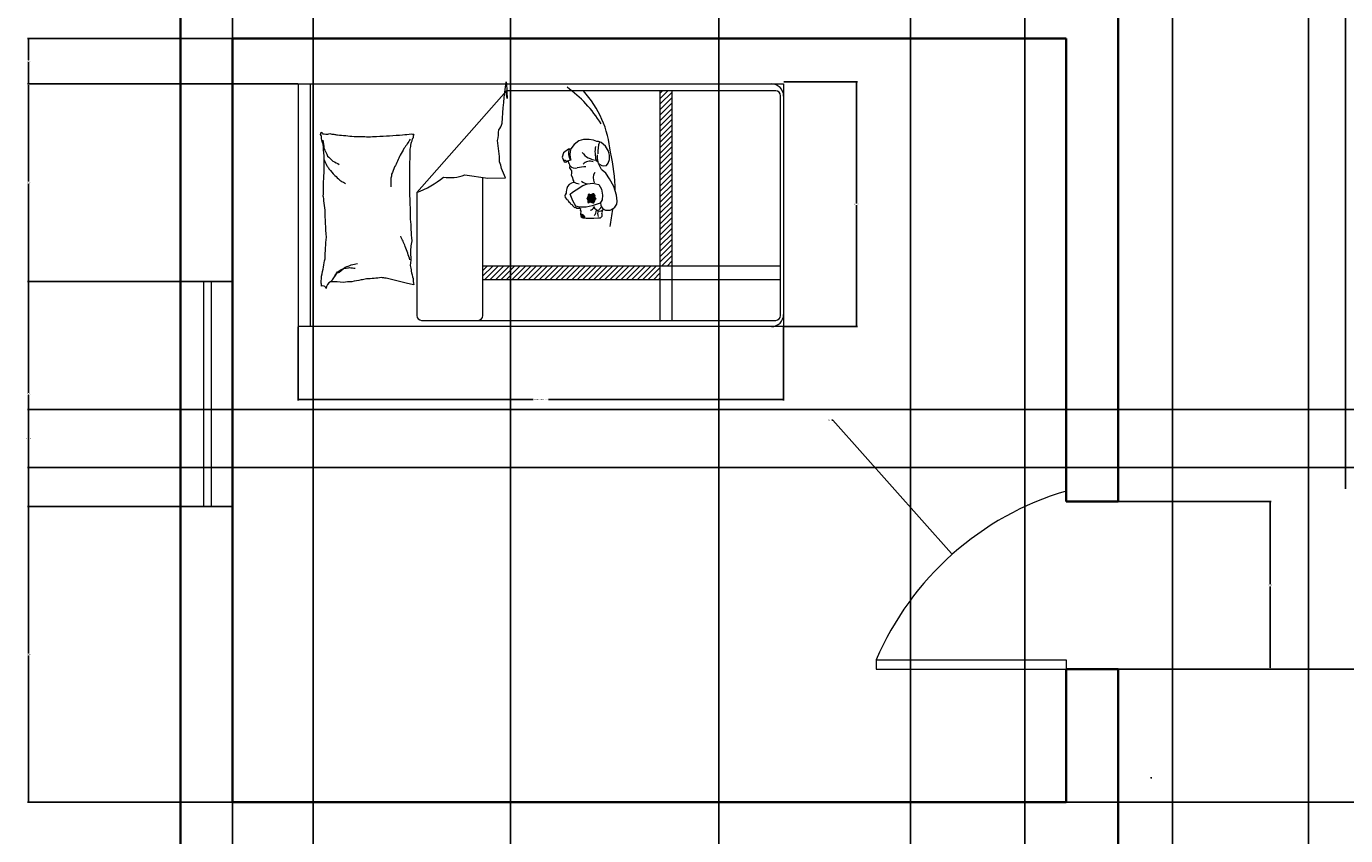
# Model space of a CAD drawing. Units: inches. Extents: x -20 to 351, y -512 to 63.
# Tile 2 of 5: x -20 to 208, y -328 to -188. Entities that reach past the tile are written whole.
import ezdxf

# ---------------------------------------------------------------- set-up
doc = ezdxf.new("R2010")
doc.units = ezdxf.units.IN
doc.header["$MEASUREMENT"] = 0
for name, color, linetype, lineweight in [('A-ANNO-DIMS', 2, 'Continuous', 18), ('A-DOOR', 3, 'Continuous', 18), ('A-FURN', 30, 'Continuous', 18), ('A-GLAZ', 4, 'Continuous', 18), ('A-WALL', 7, 'Continuous', 35)]:
    doc.layers.add(name, color=color, linetype=linetype, lineweight=lineweight)
doc.styles.get("Standard").update_dxf_attribs({"font": 'arial.ttf'})
doc.dimstyles.get("Standard").update_dxf_attribs({"dimtxt": 0.18, "dimasz": 0.18, "dimexe": 0.18, "dimexo": 0.0625, "dimgap": 0.09, "dimtad": 0, "dimtih": 1, "dimtoh": 1, "dimdec": 4, "dimzin": 0, "dimdsep": 46, "dimtxsty": 'Standard', "dimcen": 0.09, "dimadec": 0, "dimazin": 0, "dimtfac": 1, "dimtdec": 4, "dimtofl": 0, "dimtmove": 0, "dimatfit": 3, "dimfxl": 1, "dimtolj": 1, "dimtzin": 0, "dimarcsym": 0})
pattern_1 = [(135, (-420.77409, 493.76136), (-0.08072188, -0.08072188), [])]

# ---------------------------------------------------------------- blocks, each defined once
blk = doc.blocks.new('BED-SINGLE')
h = blk.add_hatch()
h.set_pattern_fill('ANSI31', color=256, scale=0.209657, angle=90, style=0)
h.set_pattern_definition([(225, (-28.8794, 49.6857), (-0.4706923, 0.4706923), [])])
h.paths.add_polyline_path([(62.56, 8.11), (62.56, 10.46), (31.92, 10.46), (31.92, 8.11)])
h.paths.add_polyline_path([(64.62, 10.46), (64.62, 40.74), (62.56, 40.74), (62.56, 10.46)])
h = blk.add_hatch()
h.set_pattern_fill('ANSI31', color=256, scale=0.913264, angle=90, style=0)
h.set_pattern_definition(pattern_1)
h.paths.add_polyline_path([(51.28, 22.35), (51.3, 22.58), (51.22, 22.8), (51.07, 22.92), (50.9, 22.92), (50.65, 22.81), (50.46, 22.77), (50.38, 22.84), (50.26, 22.89), (50.12, 22.84), (50.1, 22.73), (50.1, 22.6), (50.04, 22.43), (49.91, 22.22), (49.88, 22.16), (50.03, 21.91), (50.07, 21.8), (50.04, 21.63), (50.02, 21.51), (50.13, 21.39), (50.25, 21.43), (50.34, 21.55), (50.56, 21.53), (50.93, 21.38), (51.11, 21.41), (51.13, 21.53), (51.16, 21.62), (51.25, 21.7), (51.25, 21.79), (51.3, 21.95), (51.4, 22.06), (51.46, 22.11), (51.37, 22.18)])
h = blk.add_hatch()
h.set_pattern_fill('ANSI31', color=256, scale=0.913264, angle=90, style=0)
h.set_pattern_definition(pattern_1)
h.paths.add_polyline_path([(48.8, 19.38), (48.81, 19.17), (48.88, 18.99), (49.05, 18.85), (49.19, 18.79), (49.55, 18.75, 0.479357)])
for p, q in [((0, 41.93), (83.86, 41.93)), ((83.86, 41.93), (83.86, 0)), ((20.48, 23.17), (35.99, 40.74)), ((82.51, 40.74), (35.99, 40.74)), ((62.56, 1.08), (62.56, 40.74)), ((64.62, 1.08), (64.62, 40.74)), ((83.35, 1.92), (83.35, 39.9)), ((31.92, 1.92), (31.92, 25.76)), ((20.48, 23.17), (20.48, 1.92)), ((83.86, 0), (0, 0)), ((21.32, 1.08), (82.51, 1.08))]:
    blk.add_line(p, q)
for points in [[(0, 41.93), (0, 0)], [(2.1, 0), (2.1, 41.93)], [(49.88, 18.74), (50.44, 18.72), (51.09, 18.75), (51.78, 18.78), (51.99, 18.81), (52.24, 18.82), (52.5, 19.09), (52.51, 19.35), (52.46, 19.55), (52.59, 19.75), (52.54, 19.93), (52.68, 20.27), (52.85, 20.24), (53.09, 20.11), (53.92, 20.14), (54.4, 20.39), (54.7, 20.65), (55.03, 21.16), (55.11, 21.69), (54.99, 22.73), (54.51, 24.21), (53.78, 25.53), (53.17, 26.52), (52.53, 27.05), (52.38, 27.16), (51.98, 27.94), (51.97, 28.02), (52.04, 28.1), (52.44, 27.84), (52.72, 27.76), (53.28, 27.82), (53.58, 28.27), (53.78, 28.87), (53.81, 29.61), (53.61, 30.34), (53.08, 31.16), (52.32, 31.81), (51.86, 31.98), (51.61, 32), (51.05, 32.23), (50.29, 32.34), (49.27, 32.34), (48.48, 32.12), (47.69, 31.5), (47.1, 30.74), (46.7, 30.65), (45.83, 30.03), (45.63, 29.27), (45.94, 28.45), (46.23, 28.39), (46.51, 28.63), (46.59, 28.65), (46.7, 28.38), (46.79, 28.19), (46.84, 28.15), (46.88, 27.91), (46.94, 27.83), (46.9, 27.43), (47.08, 27.07), (47.21, 26.95), (47.22, 26.46), (47.16, 26.24), (47.34, 25.81), (47.42, 25.77), (47.46, 25.38), (47.62, 25.1), (47.53, 24.92), (47.25, 24.78), (46.82, 24.56), (46.52, 24.21), (46.42, 23.85), (46.36, 23.64), (46.33, 23.32), (46.29, 23.08), (46.15, 22.79), (46.09, 22.63), (46.1, 22.34), (46.39, 21.98), (46.55, 21.94), (46.69, 21.61), (46.82, 21.43), (46.98, 21.37), (47.06, 21.28), (47.13, 21.18), (47.37, 21.06), (47.42, 21.02), (47.42, 20.94), (47.65, 20.72), (47.76, 20.61), (47.94, 20.63), (48.13, 20.48), (48.29, 20.49), (48.59, 20.46), (48.72, 20.43), (48.78, 20.4), (48.76, 20.33), (48.74, 20.13), (48.82, 19.97), (48.83, 19.89), (48.79, 19.52), (48.81, 19.17), (48.88, 18.99), (49.05, 18.85), (49.19, 18.79), (49.73, 18.74), (49.88, 18.74)], [(47.98, 20.81), (47.46, 21.73), (46.99, 22.87), (47.37, 23.23), (48.03, 23.64), (49.19, 24.37), (50.01, 24.7), (50.89, 24.79), (51.92, 24.54), (52.4, 23.78), (52.6, 22.7), (52.51, 21.89), (52.18, 21.31), (50.82, 20.9), (49.74, 20.66), (48.6, 20.63), (47.98, 20.81)], [(49.88, 22.16), (50.03, 21.91), (50.07, 21.8), (50.04, 21.63), (50.02, 21.51), (50.13, 21.39), (50.25, 21.43), (50.34, 21.55), (50.56, 21.53), (50.93, 21.38), (51.11, 21.41), (51.13, 21.53), (51.16, 21.62), (51.25, 21.7), (51.25, 21.79), (51.3, 21.95), (51.4, 22.06), (51.46, 22.11), (51.37, 22.18), (51.28, 22.35), (51.3, 22.58), (51.22, 22.8), (51.07, 22.92), (50.9, 22.92), (50.65, 22.81), (50.46, 22.77), (50.38, 22.84), (50.26, 22.89), (50.12, 22.84), (50.1, 22.73), (50.1, 22.6), (50.04, 22.43), (49.91, 22.22), (49.88, 22.16)], [(83.35, 10.46), (31.92, 10.46)], [(83.35, 8.11), (31.92, 8.11)]]:
    blk.add_lwpolyline(points)
for points in [[(35.81, 25.72, 0.027362), (35.12, 27.33, 0.040834), (34.81, 28.47, 0.038441), (34.42, 32.14, 0.076528), (34.64, 34, 0.103649), (35.24, 35.15, -0.018778), (35.94, 42.28, -0.024037), (36.09, 39.44, -0.052315), (35.99, 40.74)], [(5.6, 7.76, 0.263368), (4.81, 6.59, 0.494818), (4.03, 6.97, 0.049225), (3.96, 7.71, 0.036831), (4.03, 8.71, 0.031893), (4.37, 10.3, -0.035782), (4.66, 11.72, -0.032941), (4.91, 15.48, -0.026564), (4.66, 20.14, -0.017905), (4.44, 21.72, 0.033397), (4.34, 22.56, 0.03204), (4.37, 24.12, -0.018442), (4.5, 26.82, -0.010837), (4.47, 29.53, -0.014624), (4.34, 31.54, -0.111249), (4.04, 32.49, 0.153708), (3.87, 33.19, 0.076444), (3.94, 33.51, 0.215512), (4.03, 33.59, 0.585858), (4.16, 33.48, -0.363489), (4.26, 33.27, -0.191716), (4.75, 33.27, 0.129675), (5.45, 33.35, 0.01735), (6.15, 33.23, -0.019326), (6.78, 33.12, -0.018818), (9.65, 32.84, -0.021828), (12.13, 32.8, -0.006204), (13.55, 32.86, -0.001963), (18.04, 33.12, -0.028341), (19.55, 33.29, 0.117014), (19.92, 33.27, 0.36606), (19.96, 33.21, 0.03973), (19.84, 32.64, 0.048309), (19.62, 32.07, -0.062981), (19.45, 31.62, -0.04058), (19.31, 30.64, -0.014345), (19.22, 27.84, -0.005484), (19.25, 22.58, -0.007153), (19.37, 18.55, -0.008762), (19.49, 16.76, 0.008153), (19.61, 14.85, 0.06251), (19.42, 12.45, -0.078669), (19.34, 10.54, -0.047825), (19.54, 9.6, 0.034494), (19.84, 8.31, 0.023571), (19.97, 7.25, 0.510228), (19.92, 7.21), (18.66, 7.52), (15.2, 8.39, -0.073041), (14.38, 8.47, -0.023305), (11.82, 8.23, -0.018299), (10.86, 8.06, 0.01097), (9.27, 7.75, 0.042281), (7.83, 7.63, 0.027201), (5.59, 7.75)], [(4.26, 32.24, -0.088153), (4.41, 30.79, -0.088153), (5.05, 29.48, -0.077547), (5.96, 28.58, -0.077547), (7.1, 27.99)], [(19.37, 32.4, -0.016108), (18.27, 30.77, -0.024599), (17.64, 29.64, -0.009477), (16.66, 27.59, -0.015937), (16.15, 26.34, -0.072521), (16, 25.65, -0.033339), (15.99, 24.13)], [(4.5, 28.8, -0.027842), (4.95, 27.81, -0.048685), (5.29, 27.28, -0.023666), (6.31, 26.11, -0.031223), (7.18, 25.31, -0.046801), (7.5, 25.1, -0.023191), (8.2, 24.76)], [(20.48, 23.17, 0.085272), (25.1, 25.83, 0.124044), (28.77, 26.21), (32.77, 25.64), (35.81, 25.72)], [(19.31, 11.55, -0.009729), (18.93, 12.7, -0.009729), (18.51, 13.82, -0.007971), (18.13, 14.74, -0.007971), (17.72, 15.64)], [(5.6, 7.75, 0.077379), (6.66, 9.21, 0.077379), (8.12, 10.28, 0.047525), (9.15, 10.7, 0.047525), (10.25, 10.91)], [(6.27, 8.86, 0.05369), (6.82, 9.46, 0.070312), (7.33, 9.8, 0.015448), (7.69, 9.96, 0.013244), (8.12, 10.11, 0.082127), (8.88, 10.24, 0.064164), (9.85, 10.11)]]:
    blk.add_lwpolyline(points, format="xyb")
for centre, radius, start, end in [((33.6, 23.46), 22.04, 31.7708, 54.3375), ((81.77, 39.84), 2.1, 0, 90), ((35.62, 28.39), 18.42, 5.4641, 42.1092), ((82.51, 39.9), 0.839, 0, 90), ((48.38, 29.88), 1.69, 151.149, 221.3836), ((49.8, 29.77), 2.87, 160.3319, 200.5181), ((51.72, 32.02), 3.26, 215.9219, 265.4055), ((57.03, 30.22), 5.75, 171.0084, 194.554), ((54.62, 29.31), 2.97, 172.9692, 196.7988), ((56.22, 30.19), 4.47, 157.6837, 184.5902), ((27.13, 23.57), 27.62, 359.7962, 13.7616), ((46.52, 29.27), 0.673, 218.3031, 258.9374), ((47.06, 28.21), 0.555, 83.9542, 141.018), ((47.86, 28.52), 1.15, 217.108, 288.2435), ((49.63, 21.97), 5.63, 89.2848, 104.5089), ((50.34, 27.01), 1.56, 67.4286, 136.0363), ((50.26, 27.3), 1.9, 23.4063, 50.8909), ((50.11, 26.41), 1.71, 226.7949, 266.7156), ((52.75, 25.69), 1.78, 147.515, 207.2356), ((50.24, 30.81), 6.38, 245.3415, 254.4913), ((50.34, 21.04), 0.905, 279.9605, 331.843), ((52.62, 21.72), 1.86, 210.5886, 253.4912), ((51.62, 20.94), 0.779, 295.2148, 339.8011), ((53.63, 21.39), 1.39, 182.1498, 236.1783), ((48.92, 18.76), 0.631, 359.0987, 101.5429), ((50.37, 20.09), 1.16, 309.7451, 1.7337), ((53.53, 19.57), 1.79, 164.8422, 197.2397), ((52.13, 20.47), 0.53, 266.1994, 319.0666), ((12.56, 24.85), 42.04, 349.6217, 353.7472), ((21.32, 1.92), 0.839, 180, 270), ((31.08, 1.92), 0.839, 270, 0), ((81.77, 2.1), 2.1, 270, 0), ((82.51, 1.92), 0.839, 270, 0)]:
    blk.add_arc(centre, radius, start, end)
blk = doc.blocks.new('*D5')
at = {"layer": 'A-ANNO-DIMS', "color": 0, "lineweight": -2, "transparency": 16777216}
for p, q in [((26.62, -239.81), (26.62, -252.51)), ((110.48, -239.81), (110.48, -252.51)), ((26.8, -252.33), (67.23, -252.33)), ((110.3, -252.33), (69.87, -252.33))]:
    blk.add_line(p, q, dxfattribs=at)
at = {"layer": 'A-ANNO-DIMS', "color": 0, "transparency": 16777216}
for points in [[(26.8, -252.3), (26.8, -252.36), (26.62, -252.33)], [(110.3, -252.3), (110.3, -252.36), (110.48, -252.33)]]:
    blk.add_solid(points, dxfattribs=at)
at = {"layer": 'Defpoints', "color": 0, "transparency": 16777216}
for p in [(26.62, -239.75), (110.48, -239.75), (110.48, -252.33)]:
    blk.add_point(p, dxfattribs=at)
at = {"layer": 'A-ANNO-DIMS', "color": 0, "transparency": 16777216, "insert": (68.55, -252.33), "char_height": 0.18, "attachment_point": 5}
blk.add_mtext('\\A1;SINGLE BED 84 TYP.', dxfattribs=at)
blk = doc.blocks.new('*D6')
at = {"layer": 'A-ANNO-DIMS', "color": 0, "lineweight": -2, "transparency": 16777216}
for p, q in [((110.54, -197.47), (123.24, -197.47)), ((123.06, -197.65), (123.06, -218.43)), ((123.06, -239.57), (123.06, -218.79)), ((110.54, -239.75), (123.24, -239.75))]:
    blk.add_line(p, q, dxfattribs=at)
at = {"layer": 'A-ANNO-DIMS', "color": 0, "transparency": 16777216}
for points in [[(123.03, -197.65), (123.09, -197.65), (123.06, -197.47)], [(123.03, -239.57), (123.09, -239.57), (123.06, -239.75)]]:
    blk.add_solid(points, dxfattribs=at)
at = {"layer": 'Defpoints', "color": 0, "transparency": 16777216}
for p in [(110.48, -197.47), (123.06, -197.47), (110.48, -239.75)]:
    blk.add_point(p, dxfattribs=at)
at = {"layer": 'A-ANNO-DIMS', "color": 0, "transparency": 16777216, "insert": (123.06, -218.61), "char_height": 0.18, "attachment_point": 5}
blk.add_mtext('\\A1;42 TYP.', dxfattribs=at)
blk = doc.blocks.new('*D9')
at = {"layer": 'A-ANNO-DIMS', "color": 0, "lineweight": -2, "transparency": 16777216}
for p, q in [((324.28, -315.88), (324.28, -512.19)), ((6.28, -485.83), (6.28, -512.19)), ((6.46, -512.01), (165, -512.01)), ((324.1, -512.01), (165.57, -512.01))]:
    blk.add_line(p, q, dxfattribs=at)
at = {"layer": 'A-ANNO-DIMS', "color": 0, "transparency": 16777216}
for points in [[(6.46, -511.98), (6.46, -512.04), (6.28, -512.01)], [(324.1, -511.98), (324.1, -512.04), (324.28, -512.01)]]:
    blk.add_solid(points, dxfattribs=at)
at = {"layer": 'Defpoints', "color": 0, "transparency": 16777216}
for p in [(324.28, -315.82), (6.28, -485.76), (324.28, -512.01)]:
    blk.add_point(p, dxfattribs=at)
at = {"layer": 'A-ANNO-DIMS', "color": 0, "transparency": 16777216, "insert": (165.28, -512.01), "char_height": 0.18, "attachment_point": 5}
blk.add_mtext('\\A1;318', dxfattribs=at)
blk = doc.blocks.new('*D17')
at = {"layer": 'A-ANNO-DIMS', "color": 0, "lineweight": -2, "transparency": 16777216}
for p, q in [((26.56, -197.82), (-20.15, -197.82)), ((-19.97, -198), (-19.97, -214.7)), ((-19.97, -231.77), (-19.97, -215.07)), ((15.22, -231.95), (-20.15, -231.95))]:
    blk.add_line(p, q, dxfattribs=at)
at = {"layer": 'A-ANNO-DIMS', "color": 0, "transparency": 16777216}
for points in [[(-20, -198), (-19.94, -198), (-19.97, -197.82)], [(-20, -231.77), (-19.94, -231.77), (-19.97, -231.95)]]:
    blk.add_solid(points, dxfattribs=at)
at = {"layer": 'Defpoints', "color": 0, "transparency": 16777216}
for p in [(26.62, -197.82), (-19.97, -231.95), (15.28, -231.95)]:
    blk.add_point(p, dxfattribs=at)
at = {"layer": 'A-ANNO-DIMS', "color": 0, "transparency": 16777216, "insert": (-19.97, -214.88), "char_height": 0.18, "attachment_point": 5}
blk.add_mtext('\\A1;34.13', dxfattribs=at)
blk = doc.blocks.new('*D18')
at = {"layer": 'A-ANNO-DIMS', "color": 0, "lineweight": -2, "transparency": 16777216}
for p, q in [((15.22, -231.95), (-20.15, -231.95)), ((-19.97, -232.13), (-19.97, -251.21)), ((-19.97, -270.65), (-19.97, -251.57)), ((15.22, -270.83), (-20.15, -270.83))]:
    blk.add_line(p, q, dxfattribs=at)
at = {"layer": 'A-ANNO-DIMS', "color": 0, "transparency": 16777216}
for points in [[(-20, -232.13), (-19.94, -232.13), (-19.97, -231.95)], [(-20, -270.65), (-19.94, -270.65), (-19.97, -270.83)]]:
    blk.add_solid(points, dxfattribs=at)
at = {"layer": 'Defpoints', "color": 0, "transparency": 16777216}
for p in [(15.28, -231.95), (-19.97, -270.83), (15.28, -270.83)]:
    blk.add_point(p, dxfattribs=at)
at = {"layer": 'A-ANNO-DIMS', "color": 0, "transparency": 16777216, "insert": (-19.97, -251.39), "char_height": 0.18, "attachment_point": 5}
blk.add_mtext('\\A1;38.88', dxfattribs=at)
blk = doc.blocks.new('*D19')
at = {"layer": 'A-ANNO-DIMS', "color": 0, "lineweight": -2, "transparency": 16777216}
for p, q in [((15.22, -270.83), (-20.15, -270.83)), ((-19.97, -271.01), (-19.97, -296.22)), ((-19.97, -321.78), (-19.97, -296.58)), ((15.22, -321.96), (-20.15, -321.96))]:
    blk.add_line(p, q, dxfattribs=at)
at = {"layer": 'A-ANNO-DIMS', "color": 0, "transparency": 16777216}
for points in [[(-20, -271.01), (-19.94, -271.01), (-19.97, -270.83)], [(-20, -321.78), (-19.94, -321.78), (-19.97, -321.96)]]:
    blk.add_solid(points, dxfattribs=at)
at = {"layer": 'Defpoints', "color": 0, "transparency": 16777216}
for p in [(15.28, -270.83), (-19.97, -321.96), (15.28, -321.96)]:
    blk.add_point(p, dxfattribs=at)
at = {"layer": 'A-ANNO-DIMS', "color": 0, "transparency": 16777216, "insert": (-19.97, -296.4), "char_height": 0.18, "attachment_point": 5}
blk.add_mtext('\\A1;51.13', dxfattribs=at)
blk = doc.blocks.new('*D35')
at = {"layer": 'A-ANNO-DIMS', "color": 0, "lineweight": -2, "transparency": 16777216}
for p, q in [((15.28, -181.03), (15.28, -512.19)), ((99.28, -181.03), (99.28, -512.19)), ((15.46, -512.01), (57.07, -512.01)), ((99.1, -512.01), (57.5, -512.01))]:
    blk.add_line(p, q, dxfattribs=at)
at = {"layer": 'A-ANNO-DIMS', "color": 0, "transparency": 16777216}
for points in [[(15.46, -511.98), (15.46, -512.04), (15.28, -512.01)], [(99.1, -511.98), (99.1, -512.04), (99.28, -512.01)]]:
    blk.add_solid(points, dxfattribs=at)
at = {"layer": 'Defpoints', "color": 0, "transparency": 16777216}
for p in [(15.28, -180.96), (99.28, -180.96), (99.28, -512.01)]:
    blk.add_point(p, dxfattribs=at)
at = {"layer": 'A-ANNO-DIMS', "color": 0, "transparency": 16777216, "insert": (57.28, -512.01), "char_height": 0.18, "attachment_point": 5}
blk.add_mtext('\\A1;84', dxfattribs=at)
blk = doc.blocks.new('*D40')
at = {"layer": 'A-ANNO-DIMS', "color": 0, "lineweight": -2, "transparency": 16777216}
for p, q in [((132.43, -125.83), (132.43, -512.19)), ((152.16, -125.83), (152.16, -512.19)), ((132.61, -512.01), (141.84, -512.01)), ((151.98, -512.01), (142.75, -512.01))]:
    blk.add_line(p, q, dxfattribs=at)
at = {"layer": 'A-ANNO-DIMS', "color": 0, "transparency": 16777216}
for points in [[(132.61, -511.98), (132.61, -512.04), (132.43, -512.01)], [(151.98, -511.98), (151.98, -512.04), (152.16, -512.01)]]:
    blk.add_solid(points, dxfattribs=at)
at = {"layer": 'Defpoints', "color": 0, "transparency": 16777216}
for p in [(132.43, -125.76), (152.16, -125.76), (132.43, -512.01)]:
    blk.add_point(p, dxfattribs=at)
at = {"layer": 'A-ANNO-DIMS', "color": 0, "transparency": 16777216, "insert": (142.3, -512.01), "char_height": 0.18, "attachment_point": 5}
blk.add_mtext('\\A1;19.727', dxfattribs=at)
blk = doc.blocks.new('*D42')
at = {"layer": 'A-ANNO-DIMS', "color": 0, "lineweight": -2, "transparency": 16777216}
for p, q in [((177.69, -125.83), (177.69, -512.19)), ((201.2, -125.83), (201.2, -512.19)), ((177.87, -512.01), (188.98, -512.01)), ((201.02, -512.01), (189.91, -512.01))]:
    blk.add_line(p, q, dxfattribs=at)
at = {"layer": 'A-ANNO-DIMS', "color": 0, "transparency": 16777216}
for points in [[(177.87, -511.98), (177.87, -512.04), (177.69, -512.01)], [(201.02, -511.98), (201.02, -512.04), (201.2, -512.01)]]:
    blk.add_solid(points, dxfattribs=at)
at = {"layer": 'Defpoints', "color": 0, "transparency": 16777216}
for p in [(177.69, -125.76), (201.2, -125.76), (201.2, -512.01)]:
    blk.add_point(p, dxfattribs=at)
at = {"layer": 'A-ANNO-DIMS', "color": 0, "transparency": 16777216, "insert": (189.45, -512.01), "char_height": 0.18, "attachment_point": 5}
blk.add_mtext('\\A1;23.516', dxfattribs=at)
blk = doc.blocks.new('*D47')
at = {"layer": 'A-ANNO-DIMS', "color": 0, "lineweight": -2, "transparency": 16777216}
for p, q in [((168.35, -269.98), (194.71, -269.98)), ((194.53, -270.16), (194.53, -284.27)), ((194.53, -298.75), (194.53, -284.64)), ((168.35, -298.93), (194.71, -298.93))]:
    blk.add_line(p, q, dxfattribs=at)
at = {"layer": 'A-ANNO-DIMS', "color": 0, "transparency": 16777216}
for points in [[(194.5, -270.16), (194.56, -270.16), (194.53, -269.98)], [(194.5, -298.75), (194.56, -298.75), (194.53, -298.93)]]:
    blk.add_solid(points, dxfattribs=at)
at = {"layer": 'Defpoints', "color": 0, "transparency": 16777216}
for p in [(168.28, -269.98), (168.28, -298.93), (194.53, -298.93)]:
    blk.add_point(p, dxfattribs=at)
at = {"layer": 'A-ANNO-DIMS', "color": 0, "transparency": 16777216, "insert": (194.53, -284.45), "char_height": 0.18, "attachment_point": 5}
blk.add_mtext('\\A1;28.955', dxfattribs=at)
blk = doc.blocks.new('*D48')
at = {"layer": 'A-ANNO-DIMS', "color": 0, "lineweight": -2, "transparency": 16777216}
for p, q in [((168.35, -298.93), (350.71, -298.93)), ((350.53, -299.11), (350.53, -310.27)), ((350.53, -321.78), (350.53, -310.63)), ((159.35, -321.96), (350.71, -321.96))]:
    blk.add_line(p, q, dxfattribs=at)
at = {"layer": 'A-ANNO-DIMS', "color": 0, "transparency": 16777216}
for points in [[(350.5, -299.11), (350.56, -299.11), (350.53, -298.93)], [(350.5, -321.78), (350.56, -321.78), (350.53, -321.96)]]:
    blk.add_solid(points, dxfattribs=at)
at = {"layer": 'Defpoints', "color": 0, "transparency": 16777216}
for p in [(168.28, -298.93), (159.28, -321.96), (350.53, -321.96)]:
    blk.add_point(p, dxfattribs=at)
at = {"layer": 'A-ANNO-DIMS', "color": 0, "transparency": 16777216, "insert": (350.53, -310.45), "char_height": 0.18, "attachment_point": 5}
blk.add_mtext('\\A1;23.03', dxfattribs=at)
blk = doc.blocks.new('*D51')
at = {"layer": 'A-ANNO-DIMS', "color": 0, "lineweight": -2, "transparency": 16777216}
for p, q in [((29.23, -468.97), (29.23, 62.67)), ((29.41, 62.49), (45.86, 62.49)), ((63.1, 62.49), (46.65, 62.49)), ((63.28, -476.7), (63.28, 62.67))]:
    blk.add_line(p, q, dxfattribs=at)
at = {"layer": 'A-ANNO-DIMS', "color": 0, "transparency": 16777216}
for points in [[(29.41, 62.52), (29.41, 62.46), (29.23, 62.49)], [(63.1, 62.52), (63.1, 62.46), (63.28, 62.49)]]:
    blk.add_solid(points, dxfattribs=at)
at = {"layer": 'Defpoints', "color": 0, "transparency": 16777216}
for p in [(63.28, 62.49), (29.23, -469.03), (63.28, -476.76)]:
    blk.add_point(p, dxfattribs=at)
at = {"layer": 'A-ANNO-DIMS', "color": 0, "transparency": 16777216, "insert": (46.26, 62.49), "char_height": 0.18, "attachment_point": 5}
blk.add_mtext('\\A1;34.06', dxfattribs=at)
blk = doc.blocks.new('*D61')
at = {"layer": 'A-ANNO-DIMS', "color": 0, "lineweight": -2, "transparency": 16777216}
for p, q in [((168.28, -269.91), (168.28, 62.67)), ((168.46, 62.49), (187.47, 62.49)), ((207.41, 62.49), (188.4, 62.49)), ((207.59, -267.77), (207.59, 62.67))]:
    blk.add_line(p, q, dxfattribs=at)
at = {"layer": 'A-ANNO-DIMS', "color": 0, "transparency": 16777216}
for points in [[(168.46, 62.52), (168.46, 62.46), (168.28, 62.49)], [(207.41, 62.52), (207.41, 62.46), (207.59, 62.49)]]:
    blk.add_solid(points, dxfattribs=at)
at = {"layer": 'Defpoints', "color": 0, "transparency": 16777216}
for p in [(207.59, 62.49), (207.59, -267.83), (168.28, -269.98)]:
    blk.add_point(p, dxfattribs=at)
at = {"layer": 'A-ANNO-DIMS', "color": 0, "transparency": 16777216, "insert": (187.94, 62.49), "char_height": 0.18, "attachment_point": 5}
blk.add_mtext('\\A1;39.305', dxfattribs=at)
blk = doc.blocks.new('*D65')
at = {"layer": 'A-ANNO-DIMS', "color": 0, "lineweight": -2, "transparency": 16777216}
for p, q in [((225.95, -254.05), (-20.15, -254.05)), ((-19.97, -254.23), (-19.97, -258.9)), ((-19.97, -263.93), (-19.97, -259.26)), ((211.25, -264.11), (-20.15, -264.11))]:
    blk.add_line(p, q, dxfattribs=at)
at = {"layer": 'A-ANNO-DIMS', "color": 0, "transparency": 16777216}
for points in [[(-20, -254.23), (-19.94, -254.23), (-19.97, -254.05)], [(-20, -263.93), (-19.94, -263.93), (-19.97, -264.11)]]:
    blk.add_solid(points, dxfattribs=at)
at = {"layer": 'Defpoints', "color": 0, "transparency": 16777216}
for p in [(-19.97, -254.05), (226.02, -254.05), (211.31, -264.11)]:
    blk.add_point(p, dxfattribs=at)
at = {"layer": 'A-ANNO-DIMS', "color": 0, "transparency": 16777216, "insert": (-19.97, -259.08), "char_height": 0.18, "attachment_point": 5}
blk.add_mtext('\\A1;10.056', dxfattribs=at)
blk = doc.blocks.new('*D69')
at = {"layer": 'A-ANNO-DIMS', "color": 0, "lineweight": -2, "transparency": 16777216}
for p, q in [((15.22, -189.96), (-20.15, -189.96)), ((-19.97, -190.14), (-19.97, -193.71)), ((-19.97, -197.64), (-19.97, -194.07)), ((26.56, -197.82), (-20.15, -197.82))]:
    blk.add_line(p, q, dxfattribs=at)
at = {"layer": 'A-ANNO-DIMS', "color": 0, "transparency": 16777216}
for points in [[(-20, -190.14), (-19.94, -190.14), (-19.97, -189.96)], [(-20, -197.64), (-19.94, -197.64), (-19.97, -197.82)]]:
    blk.add_solid(points, dxfattribs=at)
at = {"layer": 'Defpoints', "color": 0, "transparency": 16777216}
for p in [(15.28, -189.96), (-19.97, -197.82), (26.62, -197.82)]:
    blk.add_point(p, dxfattribs=at)
at = {"layer": 'A-ANNO-DIMS', "color": 0, "transparency": 16777216, "insert": (-19.97, -193.89), "char_height": 0.18, "attachment_point": 5}
blk.add_mtext('\\A1;7.855', dxfattribs=at)
blk = doc.blocks.new('*D79')
at = {"layer": 'A-ANNO-DIMS', "color": 0, "lineweight": -2, "transparency": 16777216}
for p, q in [((118.84, -255.92), (119.02, -255.92)), ((119.02, -255.92), (139.52, -278.96)), ((173.91, -317.73), (174.09, -317.73)), ((174, -317.82), (174, -317.64))]:
    blk.add_line(p, q, dxfattribs=at)
at = {"layer": 'A-ANNO-DIMS', "color": 0, "transparency": 16777216}
blk.add_solid([(139.54, -278.94), (139.5, -278.98), (139.64, -279.1)], dxfattribs=at)
at = {"layer": 'Defpoints', "color": 0, "transparency": 16777216}
for p in [(139.64, -279.1), (174, -317.73)]:
    blk.add_point(p, dxfattribs=at)
at = {"layer": 'A-ANNO-DIMS', "color": 0, "transparency": 16777216, "insert": (118.43, -255.92), "char_height": 0.18, "attachment_point": 5}
blk.add_mtext('\\A1;R51.7', dxfattribs=at)

msp = doc.modelspace()

# ---------------------------------------------------------------- linework, layer by layer
at = {"layer": 'A-DOOR'}
for p, q in [((126.4927, -297.333), (159.2844, -297.333)), ((126.4927, -297.333), (126.4927, -298.9325)), ((159.2844, -297.333), (159.2844, -298.9325)), ((126.4927, -298.9325), (159.2844, -298.9325))]:
    msp.add_line(p, q, dxfattribs=at)
msp.add_arc((174.0012, -317.7281), 51.7013, 106.537895, 156.766444, dxfattribs=at)
at = {"layer": 'A-GLAZ'}
for p, q in [((10.2504, -231.9473), (10.2504, -270.8297)), ((11.5801, -231.9473), (11.5801, -270.8297))]:
    msp.add_line(p, q, dxfattribs=at)
msp.add_lwpolyline([(6.2844, -231.9473), (15.2844, -231.9473), (15.2844, -270.8297), (6.2844, -270.8297)], close=True, dxfattribs=at)
at = {"layer": 'A-WALL'}
for p, q in [((6.2844, 36.2354), (6.2844, -476.7646)), ((168.2844, -180.9646), (168.2844, -269.9773)), ((15.2844, -189.9646), (159.2844, -189.9646)), ((15.2844, -189.9646), (15.2844, -321.9646)), ((15.2844, -189.9646), (15.2844, -321.9646)), ((159.2844, -189.9646), (159.2844, -269.9773)), ((168.2844, -269.9773), (159.2844, -269.9773)), ((159.2844, -298.9325), (168.2844, -298.9325)), ((159.2844, -298.9325), (159.2844, -321.9646)), ((168.2844, -298.9325), (168.2844, -330.9646)), ((15.2844, -321.9646), (159.2844, -321.9646))]:
    msp.add_line(p, q, dxfattribs=at)

# ---------------------------------------------------------------- block references
at = {"layer": 'A-FURN'}
msp.add_blockref('BED-SINGLE', (26.619, -239.7508), dxfattribs=at)

# ---------------------------------------------------------------- dimensions: what is measured, and where the dimension line sits
at = {"layer": 'A-ANNO-DIMS'}
for base, p1, p2, override, picture, middle in [((63.2844, 62.4854), (29.2263, -469.0292), (63.2844, -476.7646), {"dimdec": 2, "dimlfac": 1, "dimrnd": 0, "dimzin": 0, "dimdsep": 46, "dimlunit": 2}, '*D51', (46.2554, 62.4854)), ((207.5894, 62.4854), (168.2844, -269.9773), (207.5894, -267.8336), {"dimdec": 3, "dimlfac": 1, "dimrnd": 0, "dimzin": 0, "dimdsep": 46, "dimlunit": 2}, '*D61', (187.9369, 62.4854)), ((132.4341, -512.0146), (152.1609, -125.7646), (132.4341, -125.7646), {"dimdec": 3, "dimlfac": 1, "dimrnd": 0, "dimzin": 0, "dimdsep": 46, "dimlunit": 2}, '*D40', (142.2975, -512.0146)), ((201.2048, -512.0146), (177.6888, -125.7646), (201.2048, -125.7646), {"dimdec": 3, "dimlfac": 1, "dimrnd": 0, "dimzin": 0, "dimdsep": 46, "dimlunit": 2}, '*D42', (189.4468, -512.0146)), ((99.2844, -512.0146), (15.2844, -180.9646), (99.2844, -180.9646), {"dimdec": 0, "dimlfac": 1, "dimrnd": 0, "dimzin": 0, "dimdsep": 46, "dimlunit": 2}, '*D35', (57.2844, -512.0146)), ((324.2844, -512.0146), (6.2844, -485.7646), (324.2844, -315.8223), {"dimdec": 0, "dimlfac": 1, "dimrnd": 0, "dimzin": 0, "dimdsep": 46, "dimlunit": 2}, '*D9', (165.2844, -512.0146))]:
    dim = msp.add_linear_dim(base=base, p1=p1, p2=p2, dimstyle='Standard', override=override, dxfattribs=at)
    dim.commit()
    dim.dimension.update_dxf_attribs({"geometry": picture, "text_midpoint": middle})
for base, p1, p2, angle, override, picture, middle in [((-19.9656, -197.8192), (15.2844, -189.9646), (26.6189, -197.8192), 90, {"dimdec": 3, "dimlfac": 1, "dimrnd": 0, "dimzin": 0, "dimdsep": 46, "dimlunit": 2}, '*D69', (-19.9656, -193.8919)), ((-19.9656, -231.9473), (26.6189, -197.8192), (15.2844, -231.9473), 90, {"dimdec": 2, "dimlfac": 1, "dimrnd": 0, "dimzin": 0, "dimdsep": 46, "dimlunit": 2}, '*D17', (-19.9656, -214.8832)), ((-19.9656, -270.8297), (15.2844, -231.9473), (15.2844, -270.8297), 90, {"dimdec": 2, "dimlfac": 1, "dimrnd": 0, "dimzin": 0, "dimdsep": 46, "dimlunit": 2}, '*D18', (-19.9656, -251.3885)), ((-19.9656, -254.0504), (211.3088, -264.1062), (226.0172, -254.0504), 90, {"dimdec": 3, "dimlfac": 1, "dimrnd": 0, "dimzin": 0, "dimdsep": 46, "dimlunit": 2}, '*D65', (-19.9656, -259.0783)), ((-19.9656, -321.9646), (15.2844, -270.8297), (15.2844, -321.9646), 90, {"dimdec": 2, "dimlfac": 1, "dimrnd": 0, "dimzin": 0, "dimdsep": 46, "dimlunit": 2}, '*D19', (-19.9656, -296.3972)), ((194.5345, -298.9325), (168.2844, -269.9773), (168.2844, -298.9325), 270, {"dimdec": 3, "dimlfac": 1, "dimrnd": 0, "dimzin": 0, "dimdsep": 46, "dimlunit": 2}, '*D47', (194.5345, -284.4549)), ((350.5345, -321.9646), (168.2844, -298.9325), (159.2844, -321.9646), 90, {"dimdec": 2, "dimlfac": 1, "dimrnd": 0, "dimzin": 0, "dimdsep": 46, "dimlunit": 2}, '*D48', (350.5345, -310.4485))]:
    dim = msp.add_linear_dim(base=base, p1=p1, p2=p2, angle=angle, dimstyle='Standard', override=override, dxfattribs=at)
    dim.commit()
    dim.dimension.update_dxf_attribs({"geometry": picture, "text_midpoint": middle})
dim = msp.add_linear_dim(base=(123.0611, -197.4677), p1=(110.4817, -239.7505), p2=(110.4817, -197.4677), angle=90, text='<> TYP.', dimstyle='Standard', override={"dimdec": 0, "dimlfac": 1, "dimrnd": 0, "dimzin": 0, "dimdsep": 46, "dimlunit": 2}, dxfattribs=at)
dim.commit()
dim.dimension.update_dxf_attribs({"geometry": '*D6', "text_midpoint": (123.0611, -218.6091)})
dim = msp.add_linear_dim(base=(110.4817, -252.3299), p1=(26.6189, -239.7505), p2=(110.4817, -239.7505), text='SINGLE BED <> TYP.', dimstyle='Standard', override={"dimdec": 0, "dimlfac": 1, "dimrnd": 0, "dimzin": 0, "dimdsep": 46, "dimlunit": 2}, dxfattribs=at)
dim.commit()
dim.dimension.update_dxf_attribs({"geometry": '*D5', "text_midpoint": (68.5503, -252.3299)})
dim = msp.add_radius_dim(center=(174.0012, -317.7281), mpoint=(139.6402, -279.0972), dimstyle='Standard', override={"dimdec": 1, "dimlfac": 1, "dimrnd": 0, "dimzin": 0, "dimdsep": 46, "dimlunit": 2}, dxfattribs=at)
dim.commit()
dim.dimension.update_dxf_attribs({"geometry": '*D79', "text_midpoint": (118.4337, -255.9187), "dimtype": 164})

doc.saveas('drawing.dxf')
